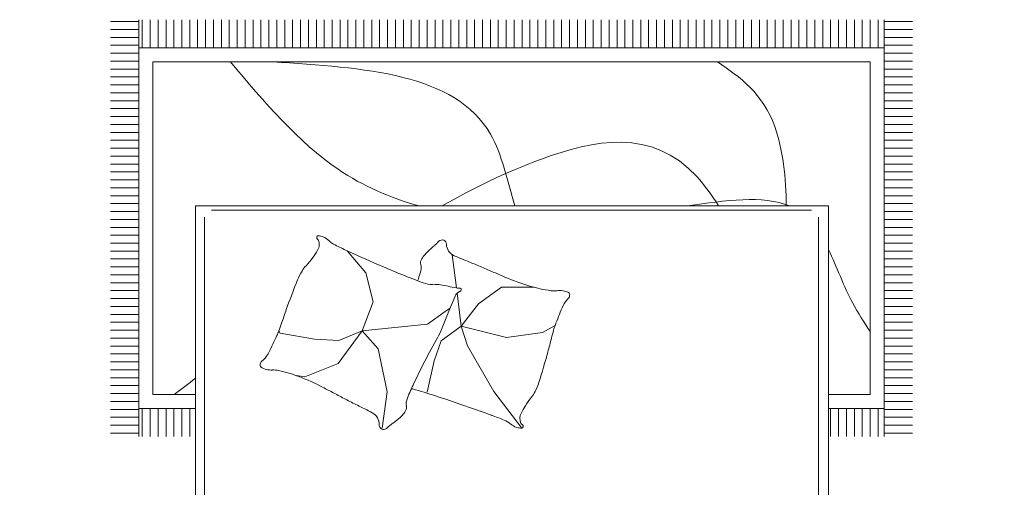
# Model space of a CAD drawing. Units: inches. Extents: x -7 to 1228, y -146 to 1091.
# Tile 61 of 88: x 443 to 530, y 614 to 655. Entities that reach past the tile are written whole.
import ezdxf

# ---------------------------------------------------------------- set-up
doc = ezdxf.new("R2010")
doc.units = ezdxf.units.IN
doc.layers.add('A-FURN', color=8, linetype='Continuous', lineweight=18)
doc.styles.add('DIM_FONT', font='SIMPLEX.shx', dxfattribs={"width": 0.8})

# ---------------------------------------------------------------- blocks, each defined once
blk = doc.blocks.new('A$C4F634EDD')
for p, q in [((0, 2.6295), (0, 2.2295)), ((0.5, 2.6295), (0, 2.6295)), ((0.5, 2.6295), (2.3, 2.6295)), ((0.5, 0.5295), (0.5, 2.6295)), ((0.5, 2.2295), (0.5, 2.6295)), ((2.3, 2.6295), (2.3, 0.5295)), ((2.3, 2.6295), (2.8, 2.6295)), ((2.3, 2.2295), (2.3, 2.6295)), ((2.8, 2.6295), (2.8, 2.2295)), ((0.5, 2.5771), (2.3, 2.5771)), ((2.392, 2.5115), (2.5692, 2.5765)), ((2.5692, 2.5765), (2.574, 2.5743)), ((0.2457, 2.5697), (0.2457, 2.4733)), ((2.4985, 2.5445), (2.5516, 2.564)), ((2.5062, 2.5454), (2.5487, 2.561)), ((2.5483, 2.5347), (2.5487, 2.561)), ((2.5487, 2.561), (2.5571, 2.56)), ((2.5615, 2.5536), (2.5514, 2.5318)), ((2.5516, 2.564), (2.5637, 2.5584)), ((2.5571, 2.56), (2.5615, 2.5536)), ((2.5615, 2.5536), (2.5791, 2.5058)), ((2.5637, 2.5584), (2.6418, 2.3458)), ((2.574, 2.5743), (2.6638, 2.3298)), ((2.4842, 2.5232), (2.47, 2.518)), ((2.4862, 2.5179), (2.4842, 2.5232)), ((2.4946, 2.5331), (2.4985, 2.5445)), ((2.5734, 2.3187), (2.4946, 2.5331)), ((2.5062, 2.5454), (2.5004, 2.5392)), ((2.5004, 2.5392), (2.5013, 2.5315)), ((2.5013, 2.5315), (2.5188, 2.4836)), ((2.5013, 2.5315), (2.5231, 2.5214)), ((2.5235, 2.5256), (2.5062, 2.5454)), ((2.5231, 2.5214), (2.5235, 2.5256)), ((2.5523, 2.4417), (2.5231, 2.5214)), ((2.5483, 2.5347), (2.5235, 2.5256)), ((2.5514, 2.5318), (2.5483, 2.5347)), ((2.5807, 2.4521), (2.5514, 2.5318)), ((2.3898, 2.5066), (2.392, 2.5115)), ((2.4795, 2.2621), (2.3898, 2.5066)), ((2.412, 2.5007), (2.4634, 2.5196)), ((2.4361, 2.4352), (2.412, 2.5007)), ((2.4634, 2.5196), (2.4875, 2.454)), ((2.47, 2.518), (2.472, 2.5127)), ((2.472, 2.5127), (2.4862, 2.5179)), ((2.4881, 2.5126), (2.4739, 2.5074)), ((2.4739, 2.5074), (2.4759, 2.502)), ((2.4759, 2.502), (2.4901, 2.5073)), ((2.492, 2.5019), (2.4778, 2.4967)), ((2.4778, 2.4967), (2.4798, 2.4914)), ((2.4798, 2.4914), (2.494, 2.4966)), ((2.4901, 2.5073), (2.4881, 2.5126)), ((2.494, 2.4966), (2.492, 2.5019)), ((2.5788, 2.4956), (2.5767, 2.4848)), ((2.5791, 2.5058), (2.5788, 2.4956)), ((2.4959, 2.4913), (2.4817, 2.4861)), ((2.4817, 2.4861), (2.4837, 2.4808)), ((2.4837, 2.4808), (2.4979, 2.486)), ((2.4998, 2.4807), (2.4856, 2.4755)), ((2.4856, 2.4755), (2.4876, 2.4702)), ((2.4876, 2.4702), (2.5018, 2.4754)), ((2.5037, 2.47), (2.4895, 2.4648)), ((2.4895, 2.4648), (2.4915, 2.4595)), ((2.4915, 2.4595), (2.5057, 2.4647)), ((2.4979, 2.486), (2.4959, 2.4913)), ((2.5018, 2.4754), (2.4998, 2.4807)), ((2.5057, 2.4647), (2.5037, 2.47)), ((2.5188, 2.4836), (2.5256, 2.4761)), ((2.5256, 2.4761), (2.5342, 2.4692)), ((2.5342, 2.4692), (2.5405, 2.4574)), ((2.5767, 2.4848), (2.5795, 2.4717)), ((2.5795, 2.4717), (2.586, 2.454)), ((2.4875, 2.454), (2.4361, 2.4352)), ((2.5405, 2.4574), (2.547, 2.4397)), ((2.5594, 2.4061), (2.547, 2.4397)), ((2.5523, 2.4417), (2.5875, 2.346)), ((2.5807, 2.4521), (2.6158, 2.3564)), ((2.5984, 2.4204), (2.586, 2.454)), ((0.0957, 2.4197), (0.192, 2.4197)), ((0.2994, 2.4197), (0.3957, 2.4197)), ((2.4457, 2.4146), (2.4563, 2.4185)), ((2.4496, 2.4039), (2.4457, 2.4146)), ((2.4563, 2.4185), (2.4602, 2.4078)), ((2.4634, 2.4211), (2.474, 2.425)), ((2.4673, 2.4104), (2.4634, 2.4211)), ((2.4779, 2.4143), (2.4673, 2.4104)), ((2.474, 2.425), (2.4779, 2.4143)), ((2.4811, 2.4276), (2.4917, 2.4315)), ((2.485, 2.4169), (2.4811, 2.4276)), ((2.4956, 2.4208), (2.485, 2.4169)), ((2.4883, 2.4081), (2.4989, 2.412)), ((2.4922, 2.3975), (2.4883, 2.4081)), ((2.4917, 2.4315), (2.4956, 2.4208)), ((2.4989, 2.412), (2.5028, 2.4014)), ((2.6047, 2.4086), (2.5984, 2.4204)), ((2.6133, 2.4017), (2.6047, 2.4086)), ((2.4602, 2.4078), (2.4496, 2.4039)), ((2.4528, 2.3951), (2.4635, 2.399)), ((2.4567, 2.3844), (2.4528, 2.3951)), ((2.4674, 2.3883), (2.4567, 2.3844)), ((2.4635, 2.399), (2.4674, 2.3883)), ((2.4706, 2.4016), (2.4812, 2.4055)), ((2.4745, 2.3909), (2.4706, 2.4016)), ((2.4851, 2.3949), (2.4745, 2.3909)), ((2.4777, 2.3821), (2.4883, 2.386)), ((2.4816, 2.3715), (2.4777, 2.3821)), ((2.4812, 2.4055), (2.4851, 2.3949)), ((2.4883, 2.386), (2.4922, 2.3754)), ((2.5028, 2.4014), (2.4922, 2.3975)), ((2.4954, 2.3886), (2.5061, 2.3925)), ((2.4993, 2.378), (2.4954, 2.3886)), ((2.51, 2.3819), (2.4993, 2.378)), ((2.5061, 2.3925), (2.51, 2.3819)), ((2.5238, 2.3769), (2.538, 2.3821)), ((2.538, 2.3821), (2.5419, 2.3715)), ((2.5622, 2.393), (2.5594, 2.4061)), ((2.5598, 2.372), (2.5601, 2.3822)), ((2.5601, 2.3822), (2.5622, 2.393)), ((2.6201, 2.3941), (2.6133, 2.4017)), ((2.6376, 2.3463), (2.6201, 2.3941)), ((2.6499, 2.3979), (2.6397, 2.3953)), ((2.6417, 2.39), (2.6488, 2.391)), ((2.6488, 2.391), (2.6538, 2.3895)), ((2.6551, 2.397), (2.6499, 2.3979)), ((2.6538, 2.3895), (2.6596, 2.388)), ((2.6627, 2.392), (2.6551, 2.397)), ((2.6596, 2.388), (2.6626, 2.3867)), ((2.6626, 2.3867), (2.6662, 2.388)), ((2.6692, 2.394), (2.6627, 2.392)), ((2.6662, 2.388), (2.6632, 2.3828)), ((2.6632, 2.3828), (2.6736, 2.3744)), ((2.6736, 2.3944), (2.6692, 2.394)), ((2.6765, 2.391), (2.6736, 2.3944)), ((2.6742, 2.3795), (2.6765, 2.391)), ((2.6824, 2.3858), (2.6742, 2.3795)), ((2.6873, 2.3815), (2.6824, 2.3858)), ((2.6853, 2.369), (2.6873, 2.3815)), ((0.2457, 2.366), (0.2457, 2.2697)), ((2.46, 2.3756), (2.4706, 2.3795)), ((2.4639, 2.365), (2.46, 2.3756)), ((2.4745, 2.3689), (2.4639, 2.365)), ((2.4672, 2.3561), (2.4778, 2.36)), ((2.4711, 2.3455), (2.4672, 2.3561)), ((2.4706, 2.3795), (2.4745, 2.3689)), ((2.4778, 2.36), (2.4817, 2.3494)), ((2.4922, 2.3754), (2.4816, 2.3715)), ((2.4849, 2.3626), (2.4955, 2.3665)), ((2.4888, 2.352), (2.4849, 2.3626)), ((2.4994, 2.3559), (2.4888, 2.352)), ((2.4955, 2.3665), (2.4994, 2.3559)), ((2.5026, 2.3691), (2.5132, 2.373)), ((2.5065, 2.3585), (2.5026, 2.3691)), ((2.5171, 2.3624), (2.5065, 2.3585)), ((2.5132, 2.373), (2.5171, 2.3624)), ((2.5277, 2.3663), (2.5238, 2.3769)), ((2.5419, 2.3715), (2.5277, 2.3663)), ((2.5774, 2.3242), (2.5598, 2.372)), ((2.6154, 2.3522), (2.5905, 2.3431)), ((2.6158, 2.3564), (2.6154, 2.3522)), ((2.6154, 2.3522), (2.6327, 2.3324)), ((2.6376, 2.3463), (2.6158, 2.3564)), ((2.6736, 2.3744), (2.6922, 2.3593)), ((2.6946, 2.376), (2.6853, 2.369)), ((2.6922, 2.3593), (2.7051, 2.3473)), ((2.6995, 2.3713), (2.6946, 2.376)), ((2.695, 2.3603), (2.6995, 2.3713)), ((2.7031, 2.3682), (2.695, 2.3603)), ((2.7096, 2.3616), (2.7031, 2.3682)), ((2.7062, 2.351), (2.7096, 2.3616)), ((2.7147, 2.3578), (2.7062, 2.351)), ((2.7214, 2.3517), (2.7147, 2.3578)), ((0, 2.3301), (0.5, 2.3301)), ((2.8, 2.3301), (2.3, 2.3301)), ((2.4817, 2.3494), (2.4711, 2.3455)), ((2.5774, 2.3242), (2.5875, 2.346)), ((2.5818, 2.3178), (2.5774, 2.3242)), ((2.5875, 2.346), (2.5905, 2.3431)), ((2.5905, 2.3431), (2.5901, 2.3168)), ((2.5901, 2.3168), (2.6097, 2.324)), ((2.613, 2.3312), (2.6077, 2.3293)), ((2.6077, 2.3293), (2.6135, 2.3141)), ((2.6192, 2.3174), (2.613, 2.3312)), ((2.6153, 2.3261), (2.6327, 2.3324)), ((2.6369, 2.332), (2.6161, 2.3243)), ((2.6616, 2.3249), (2.6234, 2.3109)), ((2.6327, 2.3324), (2.6385, 2.3386)), ((2.6418, 2.3458), (2.6369, 2.332)), ((2.6385, 2.3386), (2.6376, 2.3463)), ((2.6638, 2.3298), (2.6616, 2.3249)), ((2.7051, 2.3473), (2.7079, 2.3475)), ((2.7079, 2.3475), (2.7079, 2.3443)), ((2.7079, 2.3443), (2.727, 2.3277)), ((2.7196, 2.34), (2.7214, 2.3517)), ((2.7286, 2.3466), (2.7196, 2.34)), ((2.727, 2.3277), (2.7512, 2.2983)), ((2.7346, 2.3423), (2.7286, 2.3466)), ((2.732, 2.3295), (2.7346, 2.3423)), ((2.7423, 2.3345), (2.732, 2.3295)), ((2.7406, 2.3172), (2.7495, 2.325)), ((2.7495, 2.325), (2.7423, 2.3345)), ((2.6172, 2.3086), (2.4844, 2.2599)), ((2.5362, 2.305), (2.5185, 2.2985)), ((2.5185, 2.2985), (2.5224, 2.2879)), ((2.5401, 2.2944), (2.5362, 2.305)), ((2.561, 2.3141), (2.5433, 2.3076)), ((2.5433, 2.3076), (2.5472, 2.297)), ((2.5472, 2.297), (2.5649, 2.3035)), ((2.5649, 2.3035), (2.561, 2.3141)), ((2.5855, 2.3131), (2.5734, 2.3187)), ((2.5901, 2.3168), (2.5818, 2.3178)), ((2.6104, 2.3222), (2.5855, 2.3131)), ((2.6135, 2.3141), (2.6244, 2.2977)), ((2.626, 2.3069), (2.6192, 2.3174)), ((2.6244, 2.2977), (2.6349, 2.2825)), ((2.6365, 2.2916), (2.626, 2.3069)), ((2.7519, 2.3218), (2.7406, 2.3172)), ((2.7512, 2.2983), (2.756, 2.2695)), ((2.7575, 2.3144), (2.7519, 2.3218)), ((2.7526, 2.3045), (2.7575, 2.3144)), ((2.7622, 2.308), (2.7526, 2.3045)), ((2.7574, 2.2924), (2.7673, 2.2997)), ((2.7673, 2.2997), (2.7622, 2.308)), ((0.5953, 2.1912), (0.616, 2.2738)), ((1.4546, 2.1912), (1.4752, 2.2738)), ((2.5114, 2.2959), (2.4936, 2.2894)), ((2.4936, 2.2894), (2.4976, 2.2788)), ((2.4976, 2.2788), (2.5153, 2.2853)), ((2.5153, 2.2853), (2.5114, 2.2959)), ((2.5224, 2.2879), (2.5401, 2.2944)), ((2.6349, 2.2825), (2.638, 2.273)), ((2.6407, 2.2834), (2.6365, 2.2916)), ((2.6399, 2.2712), (2.6374, 2.2659)), ((2.638, 2.273), (2.6399, 2.2712)), ((2.6438, 2.2739), (2.6407, 2.2834)), ((2.6519, 2.2716), (2.6438, 2.2739)), ((2.6535, 2.2628), (2.6519, 2.2716)), ((2.756, 2.2695), (2.7459, 2.2483)), ((2.7687, 2.2905), (2.7574, 2.2924)), ((2.7587, 2.279), (2.7699, 2.2828)), ((2.7708, 2.2725), (2.7587, 2.279)), ((2.7699, 2.2828), (2.7687, 2.2905)), ((2.7706, 2.2643), (2.7708, 2.2725)), ((2.4844, 2.2599), (2.4795, 2.2621)), ((2.6374, 2.2659), (2.6398, 2.257)), ((2.6398, 2.257), (2.6509, 2.259)), ((2.6509, 2.259), (2.6431, 2.2492)), ((2.6431, 2.2492), (2.6473, 2.2398)), ((2.6473, 2.2398), (2.6592, 2.2429)), ((2.6592, 2.2429), (2.6521, 2.2314)), ((2.6636, 2.2409), (2.6535, 2.2628)), ((2.6836, 2.2287), (2.6636, 2.2409)), ((2.7459, 2.2483), (2.7284, 2.2317)), ((2.7509, 2.2314), (2.7459, 2.2418)), ((2.7459, 2.2418), (2.7568, 2.2352)), ((2.7529, 2.2505), (2.7645, 2.2498)), ((2.7607, 2.2424), (2.7529, 2.2505)), ((2.7568, 2.2352), (2.7607, 2.2424)), ((2.759, 2.2637), (2.7706, 2.2643)), ((2.7676, 2.2559), (2.759, 2.2637)), ((2.7645, 2.2498), (2.7676, 2.2559)), ((0, 2.2295), (0.5, 2.2295)), ((2.8, 2.2295), (2.3, 2.2295)), ((2.6521, 2.2314), (2.6598, 2.2248)), ((2.6598, 2.2248), (2.6697, 2.2309)), ((2.6697, 2.2309), (2.6684, 2.219)), ((2.6684, 2.219), (2.6761, 2.2145)), ((2.6761, 2.2145), (2.6821, 2.2237)), ((2.6821, 2.2237), (2.6843, 2.2135)), ((2.7063, 2.2256), (2.6836, 2.2287)), ((2.6843, 2.2135), (2.6927, 2.2117)), ((2.6927, 2.2117), (2.6986, 2.222)), ((2.6986, 2.222), (2.7019, 2.2098)), ((2.7284, 2.2317), (2.7063, 2.2256)), ((2.7102, 2.2104), (2.7113, 2.2218)), ((2.7113, 2.2218), (2.7192, 2.2137)), ((2.7192, 2.2137), (2.7255, 2.2152)), ((2.7255, 2.2152), (2.7242, 2.2265)), ((2.7242, 2.2265), (2.7324, 2.2165)), ((2.7324, 2.2165), (2.7386, 2.2208)), ((2.7386, 2.2208), (2.7354, 2.2306)), ((2.7354, 2.2306), (2.7462, 2.2264)), ((2.7462, 2.2264), (2.7509, 2.2314)), ((0.5878, 2.1612), (0.5953, 2.1912)), ((1.4471, 2.1612), (1.4546, 2.1912)), ((2.7019, 2.2098), (2.7102, 2.2104)), ((1.5035, 2.141), (0.5458, 2.141)), ((1.5035, 2.141), (2.2716, 1.7136)), ((0.5258, 2.121), (0.5258, 0.5617)), ((1.576, 1.9433), (1.5624, 1.8479)), ((0.5458, 1.8684), (1.5653, 1.8684)), ((1.5624, 1.8479), (1.5641, 1.7178)), ((2.2716, 0.5617), (2.2716, 1.7136)), ((0.3386, 0), (0.3386, 1.1852)), ((0.3486, 1.1052), (0.3486, 1.1852)), ((0.3711, 1.1052), (0.3711, 1.1852)), ((0.3936, 1.1052), (0.3936, 1.1852)), ((0.4161, 1.1052), (0.4161, 1.1852)), ((0.4386, 1.1052), (0.4386, 1.1852)), ((0.4611, 1.1052), (0.4611, 1.1852)), ((0.4836, 1.1052), (0.4836, 1.1852)), ((2.3061, 1.1052), (2.3061, 1.1852)), ((2.3286, 1.1052), (2.3286, 1.1852)), ((2.3511, 1.1052), (2.3511, 1.1852)), ((2.3736, 1.1052), (2.3736, 1.1852)), ((2.3961, 1.1052), (2.3961, 1.1852)), ((2.4186, 1.1052), (2.4186, 1.1852)), ((2.4411, 1.1052), (2.4411, 1.1852)), ((2.4588, 1.1852), (2.4588, 0)), ((0.2586, 1.1753), (0.3386, 1.1753)), ((0.2586, 1.1528), (0.3386, 1.1528)), ((1.031, 1.1612), (1.0448, 1.0581)), ((1.4276, 1.1611), (1.3484, 1.0571)), ((2.4588, 1.1753), (2.5388, 1.1753)), ((2.4588, 1.1528), (2.5388, 1.1528)), ((0.2586, 1.1303), (0.3386, 1.1303)), ((2.4588, 1.1303), (2.5388, 1.1303)), ((0.2586, 1.1078), (0.3386, 1.1078)), ((0.3386, 1.1052), (0.5, 1.1052)), ((2.3, 1.1052), (2.4588, 1.1052)), ((2.4588, 1.1078), (2.5388, 1.1078)), ((0.2586, 1.0853), (0.3386, 1.0853)), ((0.3786, 1.0652), (0.5, 1.0652)), ((0.3786, 0.12), (0.3786, 1.0652)), ((2.3, 1.0652), (2.4188, 1.0652)), ((2.4188, 1.0652), (2.4188, 0.12)), ((2.4588, 1.0853), (2.5388, 1.0853)), ((0.2586, 1.0628), (0.3386, 1.0628)), ((0.2586, 1.0403), (0.3386, 1.0403)), ((1.0448, 1.0581), (1.019, 0.936)), ((1.1784, 0.9702), (1.1586, 1.0591)), ((1.3484, 1.0571), (1.2733, 0.9268)), ((2.4588, 1.0628), (2.5388, 1.0628)), ((2.4588, 1.0403), (2.5388, 1.0403)), ((0.2586, 1.0178), (0.3386, 1.0178)), ((0.8108, 1.0151), (0.7868, 1.0117)), ((0.9054, 0.9773), (0.8108, 1.0151)), ((2.4588, 1.0178), (2.5388, 1.0178)), ((0.2586, 0.9953), (0.3386, 0.9953)), ((2.4588, 0.9953), (2.5388, 0.9953)), ((0.2586, 0.9728), (0.3386, 0.9728)), ((0.9743, 0.8845), (0.9054, 0.9773)), ((1.1982, 0.9129), (1.1784, 0.9702)), ((2.4588, 0.9728), (2.5388, 0.9728)), ((0.2586, 0.9503), (0.3386, 0.9503)), ((0.2586, 0.9278), (0.3386, 0.9278)), ((1.019, 0.936), (0.9743, 0.8845)), ((1.2733, 0.9268), (1.2555, 0.8715)), ((2.4588, 0.9503), (2.5388, 0.9503)), ((2.4588, 0.9278), (2.5388, 0.9278)), ((0.2586, 0.9053), (0.3386, 0.9053)), ((0.8384, 0.9085), (0.7403, 0.8913)), ((0.9072, 0.912), (0.8384, 0.9085)), ((0.9743, 0.8845), (0.9072, 0.912)), ((1.2555, 0.8715), (1.1982, 0.9129)), ((1.2555, 0.8715), (1.384, 0.9031)), ((1.384, 0.9031), (1.4868, 0.8892)), ((2.4588, 0.9053), (2.5388, 0.9053)), ((0.2586, 0.8828), (0.3386, 0.8828)), ((0.7403, 0.8913), (0.737, 0.8849)), ((0.9743, 0.8845), (1.0052, 0.802)), ((0.9743, 0.8845), (1.16, 0.8656)), ((1.1973, 0.8853), (1.2203, 0.829)), ((1.2555, 0.8715), (1.2437, 0.7773)), ((1.2555, 0.8715), (1.3049, 0.8082)), ((1.4868, 0.8892), (1.5228, 0.8692)), ((2.4588, 0.8828), (2.5388, 0.8828)), ((0.2586, 0.8603), (0.3386, 0.8603)), ((1.16, 0.8656), (1.2099, 0.8295)), ((2.4588, 0.8603), (2.5388, 0.8603)), ((0.2586, 0.8378), (0.3386, 0.8378)), ((0.2586, 0.8153), (0.3386, 0.8153)), ((1.2099, 0.8295), (1.222, 0.8209)), ((1.2203, 0.829), (1.2381, 0.7855)), ((2.4588, 0.8378), (2.5388, 0.8378)), ((2.4588, 0.8153), (2.5388, 0.8153)), ((0.2586, 0.7928), (0.3386, 0.7928)), ((1.0052, 0.802), (0.9846, 0.7194)), ((1.3049, 0.8082), (1.3701, 0.7608)), ((2.4588, 0.7928), (2.5388, 0.7928)), ((0.2586, 0.7703), (0.3386, 0.7703)), ((1.2419, 0.7626), (1.23, 0.668)), ((1.3701, 0.7608), (1.463, 0.7608)), ((2.4588, 0.7703), (2.5388, 0.7703)), ((0.2586, 0.7478), (0.3386, 0.7478)), ((2.4588, 0.7478), (2.5388, 0.7478)), ((0.2586, 0.7253), (0.3386, 0.7253)), ((0.2586, 0.7028), (0.3386, 0.7028)), ((0.9846, 0.7194), (0.931, 0.6569)), ((2.4588, 0.7253), (2.5388, 0.7253)), ((2.4588, 0.7028), (2.5388, 0.7028)), ((0.2586, 0.6803), (0.3386, 0.6803)), ((2.4588, 0.6803), (2.5388, 0.6803)), ((0.2586, 0.6578), (0.3386, 0.6578)), ((2.4588, 0.6578), (2.5388, 0.6578)), ((0.2586, 0.6353), (0.3386, 0.6353)), ((2.4588, 0.6353), (2.5388, 0.6353)), ((0.2586, 0.6128), (0.3386, 0.6128)), ((0.2586, 0.5903), (0.3386, 0.5903)), ((2.4588, 0.6128), (2.5388, 0.6128)), ((2.4588, 0.5903), (2.5388, 0.5903)), ((0.2586, 0.5678), (0.3386, 0.5678)), ((2.4588, 0.5678), (2.5388, 0.5678)), ((0.2586, 0.5453), (0.3386, 0.5453)), ((0.5458, 0.5417), (2.2516, 0.5417)), ((2.4588, 0.5453), (2.5388, 0.5453)), ((0.2586, 0.5228), (0.3386, 0.5228)), ((2.3, 0.5295), (0.5, 0.5295)), ((2.4588, 0.5228), (2.5388, 0.5228)), ((0.2586, 0.5003), (0.3386, 0.5003)), ((0.2586, 0.4778), (0.3386, 0.4778)), ((2.4588, 0.5003), (2.5388, 0.5003)), ((2.4588, 0.4778), (2.5388, 0.4778)), ((0.2586, 0.4553), (0.3386, 0.4553)), ((2.4588, 0.4553), (2.5388, 0.4553)), ((0.2586, 0.4328), (0.3386, 0.4328)), ((2.4588, 0.4328), (2.5388, 0.4328)), ((0.2586, 0.4103), (0.3386, 0.4103)), ((2.4588, 0.4103), (2.5388, 0.4103)), ((0.2586, 0.3878), (0.3386, 0.3878)), ((0.2586, 0.3653), (0.3386, 0.3653)), ((2.4588, 0.3878), (2.5388, 0.3878)), ((2.4588, 0.3653), (2.5388, 0.3653)), ((0.2586, 0.3428), (0.3386, 0.3428)), ((2.4588, 0.3428), (2.5388, 0.3428)), ((0.2586, 0.3203), (0.3386, 0.3203)), ((2.4588, 0.3203), (2.5388, 0.3203)), ((0.2586, 0.2978), (0.3386, 0.2978)), ((2.4588, 0.2978), (2.5388, 0.2978)), ((0.2586, 0.2753), (0.3386, 0.2753)), ((0.2586, 0.2528), (0.3386, 0.2528)), ((2.4588, 0.2753), (2.5388, 0.2753)), ((2.4588, 0.2528), (2.5388, 0.2528)), ((0.2586, 0.2303), (0.3386, 0.2303)), ((2.4588, 0.2303), (2.5388, 0.2303)), ((0.2586, 0.2078), (0.3386, 0.2078)), ((2.4588, 0.2078), (2.5388, 0.2078)), ((0.2586, 0.1853), (0.3386, 0.1853)), ((2.4588, 0.1853), (2.5388, 0.1853)), ((0.2586, 0.1628), (0.3386, 0.1628)), ((0.2586, 0.1403), (0.3386, 0.1403)), ((2.4588, 0.1628), (2.5388, 0.1628)), ((2.4588, 0.1403), (2.5388, 0.1403)), ((0.2586, 0.1178), (0.3386, 0.1178)), ((2.4188, 0.12), (0.3786, 0.12)), ((2.4588, 0.1178), (2.5388, 0.1178)), ((0.2586, 0.0953), (0.3386, 0.0953)), ((2.4588, 0.0953), (2.5388, 0.0953)), ((0.2586, 0.0728), (0.3386, 0.0728)), ((2.4588, 0.08), (0.3386, 0.08)), ((0.3486, 0), (0.3486, 0.08)), ((0.3711, 0), (0.3711, 0.08)), ((0.3936, 0), (0.3936, 0.08)), ((0.4161, 0), (0.4161, 0.08)), ((0.4386, 0), (0.4386, 0.08)), ((0.4611, 0), (0.4611, 0.08)), ((0.4836, 0), (0.4836, 0.08)), ((0.5061, 0), (0.5061, 0.08)), ((0.5286, 0), (0.5286, 0.08)), ((0.5511, 0), (0.5511, 0.08)), ((0.5736, 0), (0.5736, 0.08)), ((0.5961, 0), (0.5961, 0.08)), ((0.6186, 0), (0.6186, 0.08)), ((0.6411, 0), (0.6411, 0.08)), ((0.6636, 0), (0.6636, 0.08)), ((0.6861, 0), (0.6861, 0.08)), ((0.7086, 0), (0.7086, 0.08)), ((0.7311, 0), (0.7311, 0.08)), ((0.7536, 0), (0.7536, 0.08)), ((0.7761, 0), (0.7761, 0.08)), ((0.7986, 0), (0.7986, 0.08)), ((0.8211, 0), (0.8211, 0.08)), ((0.8436, 0), (0.8436, 0.08)), ((0.8661, 0), (0.8661, 0.08)), ((0.8886, 0), (0.8886, 0.08)), ((0.9111, 0), (0.9111, 0.08)), ((0.9336, 0), (0.9336, 0.08)), ((0.9561, 0), (0.9561, 0.08)), ((0.9786, 0), (0.9786, 0.08)), ((1.0011, 0), (1.0011, 0.08)), ((1.0236, 0), (1.0236, 0.08)), ((1.0461, 0), (1.0461, 0.08)), ((1.0686, 0), (1.0686, 0.08)), ((1.0911, 0), (1.0911, 0.08)), ((1.1136, 0), (1.1136, 0.08)), ((1.1361, 0), (1.1361, 0.08)), ((1.1586, 0), (1.1586, 0.08)), ((1.1811, 0), (1.1811, 0.08)), ((1.2036, 0), (1.2036, 0.08)), ((1.2261, 0), (1.2261, 0.08)), ((1.2486, 0), (1.2486, 0.08)), ((1.2711, 0), (1.2711, 0.08)), ((1.2936, 0), (1.2936, 0.08)), ((1.3161, 0), (1.3161, 0.08)), ((1.3386, 0), (1.3386, 0.08)), ((1.3611, 0), (1.3611, 0.08)), ((1.3836, 0), (1.3836, 0.08)), ((1.4061, 0), (1.4061, 0.08)), ((1.4286, 0), (1.4286, 0.08)), ((1.4511, 0), (1.4511, 0.08)), ((1.4736, 0), (1.4736, 0.08)), ((1.4961, 0), (1.4961, 0.08)), ((1.5186, 0), (1.5186, 0.08)), ((1.5411, 0), (1.5411, 0.08)), ((1.5636, 0), (1.5636, 0.08)), ((1.5861, 0), (1.5861, 0.08)), ((1.6086, 0), (1.6086, 0.08)), ((1.6311, 0), (1.6311, 0.08)), ((1.6536, 0), (1.6536, 0.08)), ((1.6761, 0), (1.6761, 0.08)), ((1.6986, 0), (1.6986, 0.08)), ((1.7211, 0), (1.7211, 0.08)), ((1.7436, 0), (1.7436, 0.08)), ((1.7661, 0), (1.7661, 0.08)), ((1.7886, 0), (1.7886, 0.08)), ((1.8111, 0), (1.8111, 0.08)), ((1.8336, 0), (1.8336, 0.08)), ((1.8561, 0), (1.8561, 0.08)), ((1.8786, 0), (1.8786, 0.08)), ((1.9011, 0), (1.9011, 0.08)), ((1.9236, 0), (1.9236, 0.08)), ((1.9461, 0), (1.9461, 0.08)), ((1.9686, 0), (1.9686, 0.08)), ((1.9911, 0), (1.9911, 0.08)), ((2.0136, 0), (2.0136, 0.08)), ((2.0361, 0), (2.0361, 0.08)), ((2.0586, 0), (2.0586, 0.08)), ((2.0811, 0), (2.0811, 0.08)), ((2.1036, 0), (2.1036, 0.08)), ((2.1261, 0), (2.1261, 0.08)), ((2.1486, 0), (2.1486, 0.08)), ((2.1711, 0), (2.1711, 0.08)), ((2.1936, 0), (2.1936, 0.08)), ((2.2161, 0), (2.2161, 0.08)), ((2.2386, 0), (2.2386, 0.08)), ((2.2611, 0), (2.2611, 0.08)), ((2.2836, 0), (2.2836, 0.08)), ((2.3061, 0), (2.3061, 0.08)), ((2.3286, 0), (2.3286, 0.08)), ((2.3511, 0), (2.3511, 0.08)), ((2.3736, 0), (2.3736, 0.08)), ((2.3961, 0), (2.3961, 0.08)), ((2.4186, 0), (2.4186, 0.08)), ((2.4411, 0), (2.4411, 0.08)), ((2.4588, 0.0728), (2.5388, 0.0728)), ((0.2586, 0.0503), (0.3386, 0.0503)), ((2.4588, 0.0503), (2.5388, 0.0503)), ((0.2586, 0.0278), (0.3386, 0.0278)), ((0.2586, 0.0053), (0.3386, 0.0053)), ((2.4588, 0.0278), (2.5388, 0.0278)), ((2.4588, 0.0053), (2.5388, 0.0053))]:
    blk.add_line(p, q)
for radius in [0.1222, 0.0865]:
    blk.add_circle((0.2457, 2.4197), radius)
for centre, radius, start, end in [((0.5848, 2.5274), 0.0131, 101.2724, 206.5805), ((0.6036, 2.5368), 0.0342, 206.5805, 265.5998), ((0.5999, 2.4516), 0.0904, 90, 101.2724), ((0.5999, 2.3808), 0.1611, 81.5628, 90), ((0.5788, 2.2388), 0.3048, 74.256, 81.5628), ((0.7272, 2.7653), 0.2422, 254.256, 262.4531), ((0.7851, 3.2019), 0.6827, 262.4531, 270), ((0.7851, 3.5682), 1.049, 270, 276.0867), ((0.8402, 3.0514), 0.5293, 276.0867, 280.1899), ((1.1602, -8.1346), 10.6675, 90.30153, 91.21582), ((1.1169, 2.2433), 0.2897, 85.1982, 92.5386), ((1.2142, 3.4021), 0.8732, 265.1982, 269.4243), ((1.3082, 2.3102), 0.234, 110.8603, 117.2396), ((1.2204, 4.0232), 1.4943, 269.4243, 271.9079), ((1.2995, 2.4357), 0.0992, 105.9352, 126.0864), ((1.2429, 3.3501), 0.8208, 271.9079, 275.2592), ((1.2995, 2.4357), 0.0992, 85.7841, 105.9352), ((1.3132, 2.5864), 0.0539, 275.2592, 300.6513), ((1.3554, 2.5152), 0.0289, 85.6975, 120.6513), ((1.3556, 2.519), 0.0251, 68.2117, 85.6975), ((1.3739, 2.5288), 0.0156, 158.0096, 201.421), ((1.3634, 2.533), 0.00428, 78.1069, 158.0096), ((1.3288, 2.5111), 0.0328, 351.8665, 21.421), ((1.3647, 2.5395), 0.00232, 258.1069, 19.564), ((1.3637, 2.5391), 0.00342, 19.564, 68.2117), ((1.444, 2.5274), 0.0131, 101.2724, 206.5805), ((1.4628, 2.5368), 0.0342, 206.5805, 265.5998), ((1.4591, 2.4516), 0.0904, 90, 101.2724), ((1.4591, 2.3808), 0.1611, 81.5628, 90), ((1.438, 2.2388), 0.3048, 74.256, 81.5628), ((1.5865, 2.7653), 0.2422, 254.256, 262.4531), ((1.6443, 3.2019), 0.6827, 262.4531, 270), ((1.6443, 3.5682), 1.049, 270, 276.0867), ((1.4785, 15.4878), 12.9656, 271.22425, 272.05324), ((1.97, 2.3805), 0.1524, 92.5386, 100.1899), ((1.9761, 2.2433), 0.2897, 85.1982, 92.5386), ((2.0734, 3.4021), 0.8732, 265.1982, 269.4243), ((2.1674, 2.3102), 0.234, 110.8603, 117.2396), ((2.0797, 4.0232), 1.4943, 269.4243, 271.9079), ((2.1588, 2.4357), 0.0992, 105.9352, 126.0864), ((2.1021, 3.3501), 0.8208, 271.9079, 275.2592), ((2.1588, 2.4357), 0.0992, 85.7841, 105.9352), ((2.1724, 2.5864), 0.0539, 275.2592, 300.6513), ((2.2146, 2.5152), 0.0289, 85.6975, 120.6513), ((2.2149, 2.519), 0.0251, 68.2117, 85.6975), ((2.2331, 2.5288), 0.0156, 158.0096, 201.421), ((2.2226, 2.533), 0.00428, 78.1069, 158.0096), ((2.1881, 2.5111), 0.0328, 351.8665, 21.421), ((2.224, 2.5395), 0.00232, 258.1069, 19.564), ((2.2229, 2.5391), 0.00342, 19.564, 68.2117), ((1.0898, 2.4496), 0.4918, 173.7676, 180), ((0.5368, 2.3783), 0.1399, 45.0976, 62.7964), ((1.4317, 2.2032), 0.3916, 128.3886, 133.8115), ((1.2362, 2.45), 0.0768, 117.2396, 128.3886), ((1.2995, 2.4357), 0.0992, 143.8234, 161.5603), ((1.2995, 2.4357), 0.0992, 126.0864, 143.8234), ((1.1177, 2.5413), 0.246, 347.8905, 351.8665), ((1.949, 2.4496), 0.4918, 173.7676, 180), ((2.291, 2.2032), 0.3916, 128.3886, 133.8115), ((2.0954, 2.45), 0.0768, 117.2396, 128.3886), ((2.1588, 2.4357), 0.0992, 143.8234, 161.5603), ((2.1588, 2.4357), 0.0992, 126.0864, 143.8234), ((1.977, 2.5413), 0.246, 347.8905, 351.8665), ((0.5462, 2.4142), 0.0899, 41.4429, 53.7359), ((0.5741, 2.4389), 0.0526, 25.3551, 41.4429), ((0.5368, 2.3783), 0.1399, 27.3988, 45.0976), ((1.1799, 2.4341), 0.0493, 140.9651, 151.6832), ((1.3165, 2.3233), 0.2252, 133.8115, 140.9651), ((2.2605, 2.3525), 0.9131, 172.3191, 176.6313), ((1.5522, 2.448), 0.1983, 167.8905, 172.3191), ((2.0391, 2.4341), 0.0493, 140.9651, 151.6832), ((2.1757, 2.3233), 0.2252, 133.8115, 140.9651), ((3.1198, 2.3525), 0.9131, 172.3191, 176.6313), ((2.4114, 2.448), 0.1983, 167.8905, 172.3191), ((0.8019, 2.4496), 0.204, 180, 189.6844), ((0.4851, 2.3967), 0.1511, 21.8149, 25.3551), ((0.4345, 2.3765), 0.2056, 18.7799, 21.8149), ((0.576, 2.4246), 0.0562, 0, 18.7799), ((0.5368, 2.3783), 0.1399, 16.515, 27.3988), ((1.3127, 2.3625), 0.2002, 151.6832, 156.9972), ((1.6611, 2.4496), 0.204, 180, 189.6844), ((2.1719, 2.3625), 0.2002, 151.6832, 156.9972), ((1.4703, 2.5637), 0.882, 189.6844, 192.1984), ((0.5406, 2.4246), 0.0915, 345.3149, 0), ((0.5368, 2.3783), 0.1399, 5.6311, 16.515), ((2.3295, 2.5637), 0.882, 189.6844, 192.1984), ((2.0266, 2.3663), 0.6787, 176.6313, 181.6331), ((2.8858, 2.3663), 0.6787, 176.6313, 181.6331), ((0.2982, 2.3103), 0.3171, 8.0051, 12.1984), ((-0.0401, 2.2627), 0.6588, 2.6649, 8.0051), ((1.1575, 2.3103), 0.3171, 8.0051, 12.1984), ((0.8191, 2.2627), 0.6588, 2.6649, 8.0051), ((2.7128, 2.3859), 1.3652, 181.6331, 183.055), ((3.5721, 2.3859), 1.3652, 181.6331, 183.055), ((14.9657, 3.0398), 13.6356, 183.05496, 183.50486), ((15.8249, 3.0398), 13.6356, 183.05496, 183.50486), ((0.5503, 2.2902), 0.0677, 345.9548, 2.6649), ((1.4096, 2.2902), 0.0677, 345.9548, 2.6649), ((1.1303, 1.9835), 0.2721, 85.9172, 93.5552), ((1.1455, 2.197), 0.058, 69.3257, 85.9172), ((0.9871, 1.7772), 0.5066, 65.6735, 69.3257), ((0.473, 2.8815), 0.7387, 293.4844, 295.3111), ((0.6058, 0.9338), 1.4323, 63.5015, 65.6735), ((1.1054, 1.9358), 0.3126, 57.865, 63.5015), ((1.3322, 2.8815), 0.7387, 293.4844, 295.3111), ((0.473, 2.8815), 0.7387, 287.1982, 289.428), ((0.473, 2.8815), 0.7387, 289.428, 291.6577), ((0.473, 2.8815), 0.7387, 291.6577, 293.4844), ((0.8841, 1.5835), 0.7286, 54.1737, 57.865), ((1.6762, 2.2258), 0.3212, 183.5049, 189.9984), ((1.3322, 2.8815), 0.7387, 287.1982, 289.428), ((1.3322, 2.8815), 0.7387, 289.428, 291.6577), ((1.3322, 2.8815), 0.7387, 291.6577, 293.4844), ((2.5355, 2.2258), 0.3212, 183.5049, 189.9984), ((0.5887, 2.1609), 0.000917, 165.9551, 274.0829), ((0.5695, 2.4301), 0.2708, 274.0829, 279.4841), ((0.5763, 2.3896), 0.2297, 279.4841, 287.3864), ((0.6807, 2.0561), 0.1197, 96.4341, 107.3864), ((0.6836, 2.0301), 0.1459, 78.4414, 96.4341), ((0.759, 2.3985), 0.2301, 258.4414, 272.7491), ((0.7026, 3.5718), 1.4048, 272.7491, 274.6176), ((0.9136, 0.9591), 1.2165, 92.6096, 94.6176), ((1.2501, -19.8405), 22.0183, 90.37908, 91.01965), ((1.2012, -3.5404), 5.7185, 89.7135, 90.9704), ((1.224, 1.0141), 1.164, 86.426, 89.7135), ((1.2875, 2.0302), 0.1459, 77.131, 86.426), ((1.3099, 2.1283), 0.0453, 62.7159, 77.131), ((1.3658, 2.2367), 0.0767, 242.7159, 253.7788), ((1.3688, 2.247), 0.0875, 253.7788, 262.8796), ((1.3581, 2.1615), 0.00132, 262.8796, 343.3022), ((1.3409, 2.1667), 0.0193, 343.3022, 9.9984), ((1.448, 2.1609), 0.000917, 165.9551, 274.0829), ((1.4288, 2.4301), 0.2708, 274.0829, 279.4841), ((1.4355, 2.3896), 0.2297, 279.4841, 287.3864), ((1.5399, 2.0561), 0.1197, 96.4341, 107.3864), ((1.5429, 2.0301), 0.1459, 78.4414, 96.4341), ((1.6182, 2.3985), 0.2301, 258.4414, 272.7491), ((1.5619, 3.5718), 1.4048, 272.7491, 274.6176), ((1.7729, 0.9591), 1.2165, 92.6096, 94.6176), ((2.1093, -19.8405), 22.0183, 90.37908, 91.01965), ((2.0605, -3.5404), 5.7185, 89.7135, 90.9704), ((2.0833, 1.0141), 1.164, 86.426, 89.7135), ((2.1467, 2.0302), 0.1459, 77.131, 86.426), ((2.1691, 2.1283), 0.0453, 62.7159, 77.131), ((2.2251, 2.2367), 0.0767, 242.7159, 253.7788), ((2.2281, 2.247), 0.0875, 253.7788, 262.8796), ((2.2174, 2.1615), 0.00132, 262.8796, 343.3022), ((2.2001, 2.1667), 0.0193, 343.3022, 9.9984), ((0.5458, 2.121), 0.02, 90, 180), ((1.2147, 1.9017), 0.3751, 20.1488, 39.6445), ((1.3977, 1.9688), 0.1801, 351.8644, 20.1488), ((0.5458, 1.8884), 0.02, 180, 270), ((1.4194, 4.2174), 2.5158, 281.6741, 283.1904), ((2.0378, 1.5789), 0.1942, 97.7304, 103.1904), ((2.0195, 1.7137), 0.0581, 79.2724, 97.7304), ((1.2737, -2.2227), 4.0646, 77.0745, 79.2724), ((0.6102, 18.0525), 16.3521, 273.75703, 274.62393), ((2.0359, 1.0981), 0.6574, 74.0648, 77.0745), ((1.0582, 5.4638), 3.7801, 277.692, 279.495), ((1.7125, -0.0344), 1.8351, 72.2636, 74.0648), ((0.9863, 1.1494), 0.0359, 297.2902, 3.2455), ((1.0348, 1.1521), 0.0127, 51.1864, 183.2455), ((0.9991, 1.1077), 0.0697, 45.8726, 51.1864), ((1.0791, 1.1902), 0.0452, 225.8726, 232.4713), ((1.2846, 1.4577), 0.3825, 232.4713, 233.7837), ((0.6683, 0.6162), 0.6605, 52.7849, 53.7837), ((1.3469, 1.2115), 0.0792, 292.7069, 308.5854), ((1.4338, 1.1026), 0.0601, 110.3452, 128.5854), ((1.4251, 1.1259), 0.0352, 86.0516, 110.3452), ((1.4376, 1.1398), 0.0142, 126.5792, 169.5926), ((1.4273, 1.1567), 0.00443, 13.2808, 86.0516), ((1.4254, 1.1562), 0.0063, 306.5792, 13.2808), ((0.9362, 0.9689), 0.2176, 46.4776, 52.7849), ((1.0327, 1.0706), 0.0774, 35.8936, 46.4776), ((-0.4107, 5.9078), 5.0942, 289.0836, 290.1287), ((1.0543, 1.9106), 0.8371, 290.1287, 292.7069), ((1.4996, 1.1284), 0.0771, 169.5926, 177.2714), ((1.4378, 1.1314), 0.0153, 177.2714, 194.5709), ((1.4611, 1.1374), 0.0393, 194.5709, 206.8179), ((1.8575, -0.7096), 2.0162, 116.4147, 117.4999), ((-0.4173, 3.8699), 3.0972, 296.4147, 297.2902), ((1.0771, 1.1027), 0.0226, 351.9508, 35.8936), ((1.1449, 1.0931), 0.0458, 171.9508, 202.4162), ((0.2266, 4.0657), 3.145, 286.6085, 289.0836), ((1.7401, 1.2785), 0.352, 206.8179, 210.9056), ((1.6045, 1.1973), 0.194, 210.9056, 219.7005), ((3.744, -4.3336), 6.1019, 117.49986, 117.84822), ((2.032, 1.4591), 1.0054, 202.4162, 205.0529), ((1.3929, 1.0217), 0.081, 26.0735, 39.7005), ((0.5736, 1.5979), 0.6236, 290.7486, 297.4921), ((-1.8336, 6.2238), 5.8383, 297.49208, 297.84822), ((1.0922, 1.1636), 0.1166, 280.7366, 286.6085), ((1.2892, 0.9709), 0.1965, 17.8396, 26.0735), ((0.6422, 1.4168), 0.43, 282.6252, 290.7486), ((2.6493, 1.7476), 1.6868, 205.0529, 207.0884), ((-0.4304, 0.4175), 2.003, 15.2625, 17.8396), ((0.6894, 0.9832), 0.0058, 121.6917, 179.0386), ((0.7004, 0.983), 0.0168, 179.0386, 229.4914), ((0.7131, 0.9448), 0.0509, 103.0402, 121.6917), ((0.7152, 0.9361), 0.0599, 86.6119, 103.0402), ((0.7224, 1.0587), 0.063, 266.6119, 282.6252), ((0.6405, 0.9128), 0.0755, 26.3332, 49.4914), ((2.541, 1.6922), 1.5652, 207.0884, 209.936), ((-1.6775, -0.2344), 2.6619, 25.1732, 26.3332), ((-0.0881, 0.5109), 1.6481, 13.841, 15.2625), ((0.5689, 0.8213), 0.1798, 20.7081, 25.1732), ((0.9989, 0.8042), 0.2143, 22.2355, 29.936), ((2.0418, 1.0357), 0.5454, 193.841, 196.3122), ((0.2268, 0.692), 0.5454, 18.2369, 20.7081), ((1.6908, 0.933), 0.1798, 196.3122, 200.7773), ((4.0115, 1.8135), 2.6619, 200.7773, 201.9373), ((2.3102, 1.3785), 1.6481, 198.2369, 199.6584), ((2.6444, 1.4979), 2.003, 199.6584, 202.2355), ((1.6124, 0.8472), 0.0755, 201.9373, 225.0955), ((1.2594, 0.7942), 0.0231, 202.2355, 252.8133), ((1.5473, 0.7819), 0.0168, 354.6428, 45.0955), ((1.1727, 0.9313), 0.1794, 277.6784, 284.8807), ((1.2689, 0.569), 0.1955, 97.9822, 104.8807), ((1.2465, 0.729), 0.034, 85.7407, 97.9822), ((1.2497, 0.772), 0.0092, 265.7407, 289.3799), ((1.2512, 0.7678), 0.00467, 289.3799, 72.8133), ((1.6266, 0.159), 0.6236, 106.3527, 113.0962), ((1.5721, 0.3449), 0.43, 98.2293, 106.3527), ((1.5195, 0.708), 0.063, 82.216, 98.2293), ((1.5362, 0.8298), 0.0599, 262.216, 278.6443), ((1.5375, 0.8209), 0.0509, 278.6443, 297.2959), ((1.5582, 0.7808), 0.0058, 297.2959, 354.6428), ((0.9722, 0.8143), 0.1965, 202.2355, 210.4694), ((2.2689, -2.1899), 3.145, 111.0043, 113.4795), ((0.1831, 0.4093), 1.0054, 18.0203, 19.3448), ((1.1834, 0.6373), 0.1166, 98.1216, 111.0043), ((1.1763, 0.687), 0.0663, 85.4882, 98.1216), ((1.1871, 0.8241), 0.0712, 265.4882, 277.6784), ((3.6722, -4.6377), 5.8383, 113.0962, 113.45234), ((0.8727, 0.7557), 0.081, 210.4694, 224.0964), ((1.0957, 0.7061), 0.0458, 347.5549, 18.0203), ((0.5234, 2.5582), 2.0162, 292.0188, 293.104), ((-1.0798, 6.3161), 6.1019, 293.10398, 293.45234), ((0.6752, 0.5644), 0.194, 35.3015, 44.0964), ((0.5462, 0.4731), 0.352, 31.2138, 35.3015), ((3.0455, -3.9778), 5.0942, 113.4795, 114.5246), ((1.1625, 0.6914), 0.0226, 167.5549, 211.4977), ((1.2092, 0.72), 0.0774, 211.4977, 222.0817), ((2.4404, -2.1823), 3.0972, 112.0188, 112.8944), ((0.8136, 0.6351), 0.0393, 18.9668, 31.2138), ((0.8364, 0.6429), 0.0153, 1.6673, 18.9668), ((1.2784, -0.1047), 0.8371, 114.5246, 117.1028), ((1.3133, 0.814), 0.2176, 222.0817, 228.389), ((1.6074, 1.1451), 0.6605, 228.389, 229.3878), ((1.2495, 0.6379), 0.0359, 112.8944, 178.8496), ((0.8506, 0.6191), 0.0063, 130.9751, 197.6767), ((0.8488, 0.6185), 0.00443, 197.6767, 270.4475), ((0.8372, 0.6345), 0.0142, 310.9751, 353.9885), ((0.8486, 0.6493), 0.0352, 270.4475, 294.7411), ((0.7746, 0.6411), 0.0771, 353.9885, 1.6673), ((0.8382, 0.6719), 0.0601, 294.7411, 312.9813), ((0.9332, 0.57), 0.0792, 117.1028, 132.9813), ((0.9284, 0.3533), 0.3825, 48.0754, 49.3878), ((1.1538, 0.6043), 0.0452, 41.4767, 48.0754), ((1.2399, 0.6804), 0.0697, 221.4767, 226.7905), ((1.2009, 0.6389), 0.0127, 226.7905, 358.8496)]:
    blk.add_arc(centre, radius, start, end)
for points in [[(0.4393, 1.0652), (0.4595, 1.05), (0.4798, 1.0348), (0.5, 1.0195)], [(1.9003, 0.5295), (2.0065, 0.514), (2.1132, 0.4978), (2.1894, 0.5295)]]:
    blk.add_open_spline(points, degree=3)
for points, knots in [([(2.3, 0.6535), (2.3236, 0.7026), (2.3554, 0.7914), (2.4015, 0.8608), (2.4188, 0.8868)], [1893.525221, 1893.525221, 1893.525221, 1893.525221, 2051.902476, 2146.74457, 2146.74457, 2146.74457, 2146.74457]), ([(0.5992, 0.12), (0.6957, 0.2341), (0.8523, 0.4189), (1.0536, 0.5069), (1.136, 0.5295)], [0, 0, 0, 0, 432.822832, 701.445452, 701.445452, 701.445452, 701.445452]), ([(0.7187, 0.12), (0.9791, 0.1362), (1.326, 0.1577), (1.3868, 0.4574), (1.408, 0.5295)], [0, 0, 0, 0, 653.160442, 870.050857, 870.050857, 870.050857, 870.050857]), ([(1.2016, 0.5295), (1.2892, 0.479), (1.5144, 0.3684), (1.8265, 0.2994), (1.9681, 0.4992), (1.9875, 0.5295)], [936.534237, 936.534237, 936.534237, 936.534237, 1243.285375, 1683.261222, 1758.254386, 1758.254386, 1758.254386, 1758.254386]), ([(2.1796, 0.5295), (2.1798, 0.4519), (2.1548, 0.2369), (2.0487, 0.164), (1.9846, 0.12)], [2202.034493, 2202.034493, 2202.034493, 2202.034493, 2357.807635, 2594.446174, 2594.446174, 2594.446174, 2594.446174])]:
    blk.add_open_spline(points, degree=3, knots=knots)
at = {"style": 'DIM_FONT', "width": 0.8, "flags": 9}
for tag, p in [('YSIZE', (0.5, 2.6295)), ('XSIZE', (0.5, 2.6295)), ('XSIZE', (2.2985, 2.6295)), ('YSIZE', (2.2985, 2.6295))]:
    blk.add_attdef(tag, p, '', height=0.0005, dxfattribs=at)

msp = doc.modelspace()

# ---------------------------------------------------------------- block references
at = {"layer": 'A-FURN', "xscale": -30.79356024027943, "yscale": 30.79356024027943, "zscale": 30.79356024027943, "rotation": 180}
msp.add_blockref('A$C4F634EDD', (443.284, 654.972), dxfattribs=at)

doc.saveas('drawing.dxf')
